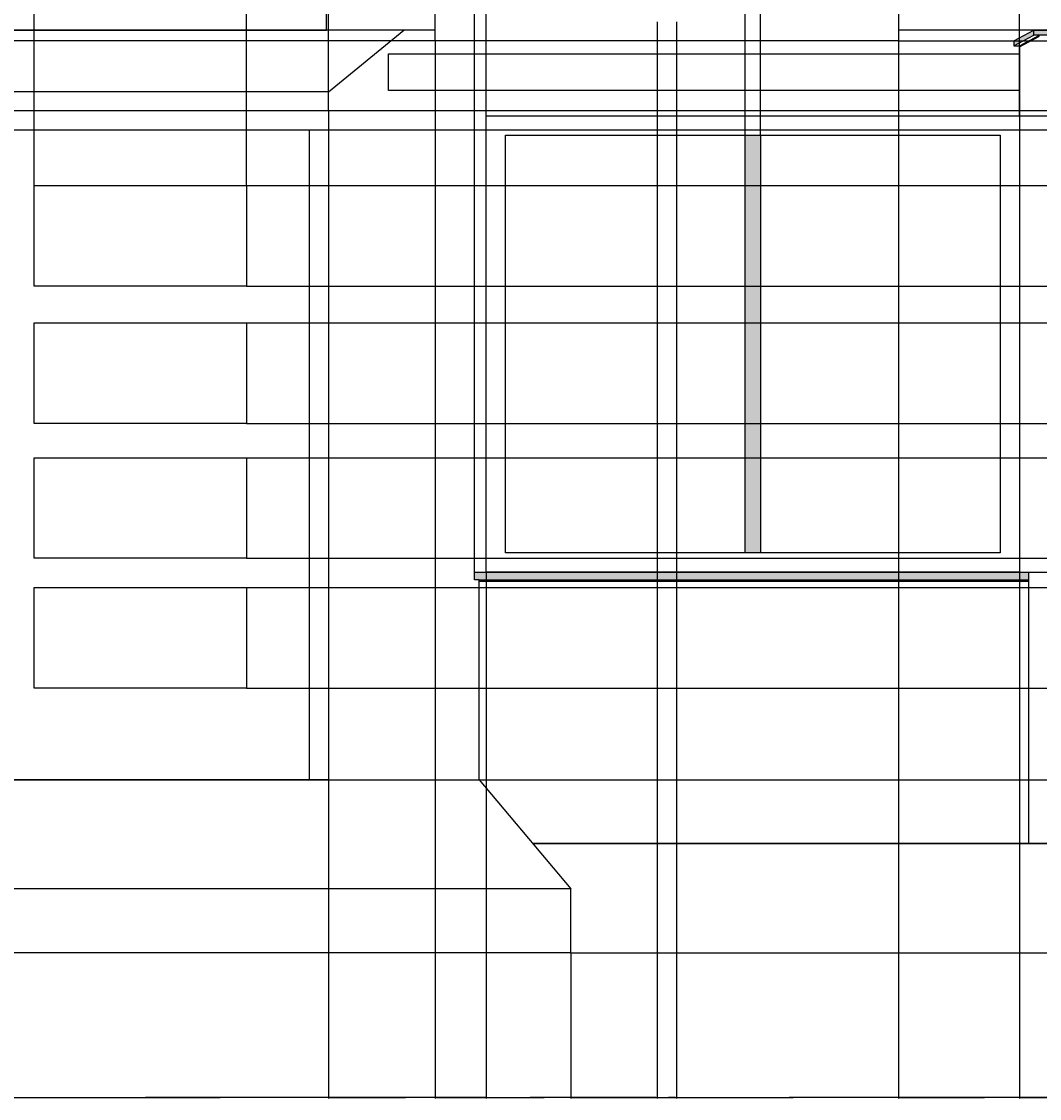
# Model space of a CAD drawing. Units: millimetres. Extents: x 171 to 1599, y 973 to 1509.
# Tile 5 of 7: x 1235 to 1445, y 973 to 1196. Entities that reach past the tile are written whole.
import ezdxf

# ---------------------------------------------------------------- set-up
doc = ezdxf.new("R2010")
doc.units = ezdxf.units.MM
for name, color, linetype, lineweight in [('A-ANNO-DIMS', 2, 'Continuous', 18), ('A-ELEV', 7, 'Continuous', 25), ('A-ELEV-FILL', 252, 'Continuous', 13)]:
    doc.layers.add(name, color=color, linetype=linetype, lineweight=lineweight)
doc.styles.get("Standard").update_dxf_attribs({"font": 'arial.ttf'})
doc.dimstyles.get("Standard").update_dxf_attribs({"dimtxt": 0.18, "dimasz": 0.18, "dimexe": 0.18, "dimexo": 0.0625, "dimgap": 0.09, "dimtad": 0, "dimtih": 1, "dimtoh": 1, "dimdec": 1, "dimzin": 0, "dimdsep": 46, "dimlunit": 3, "dimtxsty": 'Standard', "dimcen": 0.09, "dimadec": 0, "dimazin": 0, "dimtfac": 1, "dimtdec": 1, "dimtofl": 0, "dimtmove": 0, "dimatfit": 3, "dimfxl": 1, "dimtolj": 1, "dimtzin": 0, "dimarcsym": 0})

# ---------------------------------------------------------------- blocks, each defined once
blk = doc.blocks.new('*D1')
at = {"layer": 'A-ANNO-DIMS', "color": 0, "lineweight": -2, "transparency": 16777216}
for p, q in [((980.93, 1194.55), (980.93, 1508.31)), ((981.11, 1508.13), (1274.61, 1508.13)), ((1568.85, 1508.13), (1275.36, 1508.13)), ((1569.03, 1215.31), (1569.03, 1508.31))]:
    blk.add_line(p, q, dxfattribs=at)
at = {"layer": 'A-ANNO-DIMS', "color": 0, "transparency": 16777216}
for points in [[(981.11, 1508.16), (981.11, 1508.1), (980.93, 1508.13)], [(1568.85, 1508.16), (1568.85, 1508.1), (1569.03, 1508.13)]]:
    blk.add_solid(points, dxfattribs=at)
at = {"layer": 'Defpoints', "color": 0, "transparency": 16777216}
for p in [(1569.03, 1508.13), (1569.03, 1215.25), (980.93, 1194.49)]:
    blk.add_point(p, dxfattribs=at)
at = {"layer": 'A-ANNO-DIMS', "color": 0, "transparency": 16777216, "insert": (1274.98, 1508.13), "char_height": 0.18, "attachment_point": 5}
blk.add_mtext('\\A1;588.1', dxfattribs=at)
blk = doc.blocks.new('*D2')
at = {"layer": 'A-ANNO-DIMS', "color": 0, "lineweight": -2, "transparency": 16777216}
for p, q in [((1043.70287, 1478.130098), (1599.212656, 1478.130098)), ((1599.032656, 1477.950098), (1599.032656, 1240.959874)), ((1599.032656, 1003.60965), (1599.032656, 1240.599874)), ((1348.449149, 1003.42965), (1599.212656, 1003.42965))]:
    blk.add_line(p, q, dxfattribs=at)
at = {"layer": 'A-ANNO-DIMS', "color": 0, "transparency": 16777216}
for points in [[(1599.002656, 1477.950098), (1599.062656, 1477.950098), (1599.032656, 1478.130098)], [(1599.002656, 1003.60965), (1599.062656, 1003.60965), (1599.032656, 1003.42965)]]:
    blk.add_solid(points, dxfattribs=at)
at = {"layer": 'Defpoints', "color": 0, "transparency": 16777216}
for p in [(1043.64037, 1478.130098), (1599.032656, 1478.130098), (1348.386649, 1003.42965)]:
    blk.add_point(p, dxfattribs=at)
at = {"layer": 'A-ANNO-DIMS', "color": 0, "transparency": 16777216, "insert": (1599.032656, 1240.779874), "char_height": 0.18, "attachment_point": 5}
blk.add_mtext('\\A1;474.7', dxfattribs=at)
blk = doc.blocks.new('*D6')
at = {"layer": 'A-ANNO-DIMS', "color": 0, "lineweight": -2, "transparency": 16777216}
for p, q in [((1221.72, 1039.19), (1221.72, 973.25)), ((1298.24, 1039.19), (1298.24, 973.25)), ((1221.9, 973.43), (1259.59, 973.43)), ((1298.06, 973.43), (1260.37, 973.43))]:
    blk.add_line(p, q, dxfattribs=at)
at = {"layer": 'A-ANNO-DIMS', "color": 0, "transparency": 16777216}
for points in [[(1221.9, 973.46), (1221.9, 973.4), (1221.72, 973.43)], [(1298.06, 973.46), (1298.06, 973.4), (1298.24, 973.43)]]:
    blk.add_solid(points, dxfattribs=at)
at = {"layer": 'Defpoints', "color": 0, "transparency": 16777216}
for p in [(1221.72, 1039.25), (1298.24, 1039.25), (1298.24, 973.43)]:
    blk.add_point(p, dxfattribs=at)
at = {"layer": 'A-ANNO-DIMS', "color": 0, "transparency": 16777216, "insert": (1259.98, 973.43), "char_height": 0.18, "attachment_point": 5}
blk.add_mtext('\\A1;76.52', dxfattribs=at)
blk = doc.blocks.new('*D7')
at = {"layer": 'A-ANNO-DIMS', "color": 0, "lineweight": -2, "transparency": 16777216}
for p, q in [((1330.9, 1082.17), (1330.9, 973.25)), ((1298.24, 1039.19), (1298.24, 973.25)), ((1298.42, 973.43), (1314.17, 973.43)), ((1330.72, 973.43), (1314.96, 973.43))]:
    blk.add_line(p, q, dxfattribs=at)
at = {"layer": 'A-ANNO-DIMS', "color": 0, "transparency": 16777216}
for points in [[(1298.42, 973.46), (1298.42, 973.4), (1298.24, 973.43)], [(1330.72, 973.46), (1330.72, 973.4), (1330.9, 973.43)]]:
    blk.add_solid(points, dxfattribs=at)
at = {"layer": 'Defpoints', "color": 0, "transparency": 16777216}
for p in [(1330.9, 1082.23), (1298.24, 1039.25), (1330.9, 973.43)]:
    blk.add_point(p, dxfattribs=at)
at = {"layer": 'A-ANNO-DIMS', "color": 0, "transparency": 16777216, "insert": (1314.57, 973.43), "char_height": 0.18, "attachment_point": 5}
blk.add_mtext('\\A1;32.66', dxfattribs=at)
blk = doc.blocks.new('*D8')
at = {"layer": 'A-ANNO-DIMS', "color": 0, "lineweight": -2, "transparency": 16777216}
for p, q in [((1330.9, 1082.17), (1330.9, 973.25)), ((1348.39, 1003.37), (1348.39, 973.25)), ((1331.08, 973.43), (1339.26, 973.43)), ((1348.21, 973.43), (1340.03, 973.43))]:
    blk.add_line(p, q, dxfattribs=at)
at = {"layer": 'A-ANNO-DIMS', "color": 0, "transparency": 16777216}
for points in [[(1331.08, 973.46), (1331.08, 973.4), (1330.9, 973.43)], [(1348.21, 973.46), (1348.21, 973.4), (1348.39, 973.43)]]:
    blk.add_solid(points, dxfattribs=at)
at = {"layer": 'Defpoints', "color": 0, "transparency": 16777216}
for p in [(1330.9, 1082.23), (1348.39, 1003.43), (1348.39, 973.43)]:
    blk.add_point(p, dxfattribs=at)
at = {"layer": 'A-ANNO-DIMS', "color": 0, "transparency": 16777216, "insert": (1339.64, 973.43), "char_height": 0.18, "attachment_point": 5}
blk.add_mtext('\\A1;17.49', dxfattribs=at)
blk = doc.blocks.new('*D9')
at = {"layer": 'A-ANNO-DIMS', "color": 0, "lineweight": -2, "transparency": 16777216}
for p, q in [((1441.28, 1082.17), (1441.28, 973.25)), ((1348.39, 1003.37), (1348.39, 973.25)), ((1348.57, 973.43), (1394.44, 973.43)), ((1441.1, 973.43), (1395.23, 973.43))]:
    blk.add_line(p, q, dxfattribs=at)
at = {"layer": 'A-ANNO-DIMS', "color": 0, "transparency": 16777216}
for points in [[(1348.57, 973.46), (1348.57, 973.4), (1348.39, 973.43)], [(1441.1, 973.46), (1441.1, 973.4), (1441.28, 973.43)]]:
    blk.add_solid(points, dxfattribs=at)
at = {"layer": 'Defpoints', "color": 0, "transparency": 16777216}
for p in [(1441.28, 1082.23), (1348.39, 1003.43), (1441.28, 973.43)]:
    blk.add_point(p, dxfattribs=at)
at = {"layer": 'A-ANNO-DIMS', "color": 0, "transparency": 16777216, "insert": (1394.83, 973.43), "char_height": 0.18, "attachment_point": 5}
blk.add_mtext('\\A1;92.89', dxfattribs=at)
blk = doc.blocks.new('*D10')
at = {"layer": 'A-ANNO-DIMS', "color": 0, "lineweight": -2, "transparency": 16777216}
for p, q in [((1441.28, 1082.17), (1441.28, 973.25)), ((1504.77, 1026.01), (1504.77, 973.25)), ((1441.46, 973.43), (1472.63, 973.43)), ((1504.59, 973.43), (1473.42, 973.43))]:
    blk.add_line(p, q, dxfattribs=at)
at = {"layer": 'A-ANNO-DIMS', "color": 0, "transparency": 16777216}
for points in [[(1441.46, 973.46), (1441.46, 973.4), (1441.28, 973.43)], [(1504.59, 973.46), (1504.59, 973.4), (1504.77, 973.43)]]:
    blk.add_solid(points, dxfattribs=at)
at = {"layer": 'Defpoints', "color": 0, "transparency": 16777216}
for p in [(1441.28, 1082.23), (1504.77, 1026.08), (1504.77, 973.43)]:
    blk.add_point(p, dxfattribs=at)
at = {"layer": 'A-ANNO-DIMS', "color": 0, "transparency": 16777216, "insert": (1473.02, 973.43), "char_height": 0.18, "attachment_point": 5}
blk.add_mtext('\\A1;63.49', dxfattribs=at)
blk = doc.blocks.new('*D54')
at = {"layer": 'A-ANNO-DIMS', "color": 0, "lineweight": -2, "transparency": 16777216}
for p, q in [((1232.1, 1203.73), (1232.1, 973.25)), ((1320.32, 1192.2), (1320.32, 973.25)), ((1232.28, 973.43), (1275.82, 973.43)), ((1320.14, 973.43), (1276.6, 973.43))]:
    blk.add_line(p, q, dxfattribs=at)
at = {"layer": 'A-ANNO-DIMS', "color": 0, "transparency": 16777216}
for points in [[(1232.28, 973.46), (1232.28, 973.4), (1232.1, 973.43)], [(1320.14, 973.46), (1320.14, 973.4), (1320.32, 973.43)]]:
    blk.add_solid(points, dxfattribs=at)
at = {"layer": 'Defpoints', "color": 0, "transparency": 16777216}
for p in [(1232.1, 1203.79), (1320.32, 1192.27), (1320.32, 973.43)]:
    blk.add_point(p, dxfattribs=at)
at = {"layer": 'A-ANNO-DIMS', "color": 0, "transparency": 16777216, "insert": (1276.21, 973.43), "char_height": 0.18, "attachment_point": 5}
blk.add_mtext('\\A1;88.22', dxfattribs=at)
blk = doc.blocks.new('*D55')
at = {"layer": 'A-ANNO-DIMS', "color": 0, "lineweight": -2, "transparency": 16777216}
for p, q in [((1366.27, 1196.2), (1366.27, 973.25)), ((1320.32, 1192.2), (1320.32, 973.25)), ((1320.5, 973.43), (1342.9, 973.43)), ((1366.09, 973.43), (1343.69, 973.43))]:
    blk.add_line(p, q, dxfattribs=at)
at = {"layer": 'A-ANNO-DIMS', "color": 0, "transparency": 16777216}
for points in [[(1320.5, 973.46), (1320.5, 973.4), (1320.32, 973.43)], [(1366.09, 973.46), (1366.09, 973.4), (1366.27, 973.43)]]:
    blk.add_solid(points, dxfattribs=at)
at = {"layer": 'Defpoints', "color": 0, "transparency": 16777216}
for p in [(1366.27, 1196.27), (1320.32, 1192.27), (1366.27, 973.43)]:
    blk.add_point(p, dxfattribs=at)
at = {"layer": 'A-ANNO-DIMS', "color": 0, "transparency": 16777216, "insert": (1343.3, 973.43), "char_height": 0.18, "attachment_point": 5}
blk.add_mtext('\\A1;45.95', dxfattribs=at)
blk = doc.blocks.new('*D56')
at = {"layer": 'A-ANNO-DIMS', "color": 0, "lineweight": -2, "transparency": 16777216}
for p, q in [((1366.27, 1196.2), (1366.27, 973.25)), ((1370.27, 1196.2), (1370.27, 973.25)), ((1366.45, 973.43), (1367.94, 973.43)), ((1370.09, 973.43), (1368.6, 973.43))]:
    blk.add_line(p, q, dxfattribs=at)
at = {"layer": 'A-ANNO-DIMS', "color": 0, "transparency": 16777216}
for points in [[(1366.45, 973.46), (1366.45, 973.4), (1366.27, 973.43)], [(1370.09, 973.46), (1370.09, 973.4), (1370.27, 973.43)]]:
    blk.add_solid(points, dxfattribs=at)
at = {"layer": 'Defpoints', "color": 0, "transparency": 16777216}
for p in [(1366.27, 1196.27), (1370.27, 1196.27), (1370.27, 973.43)]:
    blk.add_point(p, dxfattribs=at)
at = {"layer": 'A-ANNO-DIMS', "color": 0, "transparency": 16777216, "insert": (1368.27, 973.43), "char_height": 0.18, "attachment_point": 5}
blk.add_mtext('\\A1;4.00', dxfattribs=at)
blk = doc.blocks.new('*D57')
at = {"layer": 'A-ANNO-DIMS', "color": 0, "lineweight": -2, "transparency": 16777216}
for p, q in [((1370.27, 1196.2), (1370.27, 973.25)), ((1416.22, 1192.2), (1416.22, 973.25)), ((1370.45, 973.43), (1392.85, 973.43)), ((1416.04, 973.43), (1393.64, 973.43))]:
    blk.add_line(p, q, dxfattribs=at)
at = {"layer": 'A-ANNO-DIMS', "color": 0, "transparency": 16777216}
for points in [[(1370.45, 973.46), (1370.45, 973.4), (1370.27, 973.43)], [(1416.04, 973.46), (1416.04, 973.4), (1416.22, 973.43)]]:
    blk.add_solid(points, dxfattribs=at)
at = {"layer": 'Defpoints', "color": 0, "transparency": 16777216}
for p in [(1370.27, 1196.27), (1416.22, 1192.27), (1416.22, 973.43)]:
    blk.add_point(p, dxfattribs=at)
at = {"layer": 'A-ANNO-DIMS', "color": 0, "transparency": 16777216, "insert": (1393.25, 973.43), "char_height": 0.18, "attachment_point": 5}
blk.add_mtext('\\A1;45.95', dxfattribs=at)
blk = doc.blocks.new('*D58')
at = {"layer": 'A-ANNO-DIMS', "color": 0, "lineweight": -2, "transparency": 16777216}
for p, q in [((1452.86, 1194.43), (1452.86, 973.25)), ((1416.22, 1192.2), (1416.22, 973.25)), ((1416.4, 973.43), (1434.08, 973.43)), ((1452.68, 973.43), (1435, 973.43))]:
    blk.add_line(p, q, dxfattribs=at)
at = {"layer": 'A-ANNO-DIMS', "color": 0, "transparency": 16777216}
for points in [[(1416.4, 973.46), (1416.4, 973.4), (1416.22, 973.43)], [(1452.68, 973.46), (1452.68, 973.4), (1452.86, 973.43)]]:
    blk.add_solid(points, dxfattribs=at)
at = {"layer": 'Defpoints', "color": 0, "transparency": 16777216}
for p in [(1452.86, 1194.49), (1416.22, 1192.27), (1452.86, 973.43)]:
    blk.add_point(p, dxfattribs=at)
at = {"layer": 'A-ANNO-DIMS', "color": 0, "transparency": 16777216, "insert": (1434.54, 973.43), "char_height": 0.18, "attachment_point": 5}
blk.add_mtext('\\A1;36.636', dxfattribs=at)
blk = doc.blocks.new('*D61')
at = {"layer": 'A-ANNO-DIMS', "color": 0, "lineweight": -2, "transparency": 16777216}
for p, q in [((1320.26, 1345.85), (950.75, 1345.85)), ((950.93, 1345.67), (950.93, 1269.24)), ((950.93, 1192.45), (950.93, 1268.88)), ((1320.26, 1192.27), (950.75, 1192.27))]:
    blk.add_line(p, q, dxfattribs=at)
at = {"layer": 'A-ANNO-DIMS', "color": 0, "transparency": 16777216}
for points in [[(950.9, 1345.67), (950.96, 1345.67), (950.93, 1345.85)], [(950.9, 1192.45), (950.96, 1192.45), (950.93, 1192.27)]]:
    blk.add_solid(points, dxfattribs=at)
at = {"layer": 'Defpoints', "color": 0, "transparency": 16777216}
for p in [(950.93, 1345.85), (1320.32, 1345.85), (1320.32, 1192.27)]:
    blk.add_point(p, dxfattribs=at)
at = {"layer": 'A-ANNO-DIMS', "color": 0, "transparency": 16777216, "insert": (950.93, 1269.06), "char_height": 0.18, "attachment_point": 5}
blk.add_mtext('\\A1;153.59', dxfattribs=at)
blk = doc.blocks.new('*D62')
at = {"layer": 'A-ANNO-DIMS', "color": 0, "lineweight": -2, "transparency": 16777216}
for p, q in [((1416.28, 1290.48), (1599.21, 1290.48)), ((1599.03, 1290.3), (1599.03, 1241.56)), ((1599.03, 1192.45), (1599.03, 1241.19)), ((1416.28, 1192.27), (1599.21, 1192.27))]:
    blk.add_line(p, q, dxfattribs=at)
at = {"layer": 'A-ANNO-DIMS', "color": 0, "transparency": 16777216}
for points in [[(1599, 1290.3), (1599.06, 1290.3), (1599.03, 1290.48)], [(1599, 1192.45), (1599.06, 1192.45), (1599.03, 1192.27)]]:
    blk.add_solid(points, dxfattribs=at)
at = {"layer": 'Defpoints', "color": 0, "transparency": 16777216}
for p in [(1416.22, 1290.48), (1599.03, 1290.48), (1416.22, 1192.27)]:
    blk.add_point(p, dxfattribs=at)
at = {"layer": 'A-ANNO-DIMS', "color": 0, "transparency": 16777216, "insert": (1599.03, 1241.38), "char_height": 0.18, "attachment_point": 5}
blk.add_mtext('\\A1;98.22', dxfattribs=at)
blk = doc.blocks.new('*D73')
at = {"layer": 'A-ANNO-DIMS', "color": 0, "lineweight": -2, "transparency": 16777216}
for p, q in [((1231.46, 1114.32), (1231.46, 1508.31)), ((1231.64, 1508.13), (1234.06, 1508.13)), ((1237.13, 1508.13), (1234.71, 1508.13)), ((1237.31, 1162.35), (1237.31, 1508.31))]:
    blk.add_line(p, q, dxfattribs=at)
at = {"layer": 'A-ANNO-DIMS', "color": 0, "transparency": 16777216}
for points in [[(1231.64, 1508.16), (1231.64, 1508.1), (1231.46, 1508.13)], [(1237.13, 1508.16), (1237.13, 1508.1), (1237.31, 1508.13)]]:
    blk.add_solid(points, dxfattribs=at)
at = {"layer": 'Defpoints', "color": 0, "transparency": 16777216}
for p in [(1237.31, 1508.13), (1237.31, 1162.29), (1231.46, 1114.25)]:
    blk.add_point(p, dxfattribs=at)
at = {"layer": 'A-ANNO-DIMS', "color": 0, "transparency": 16777216, "insert": (1234.38, 1508.13), "char_height": 0.18, "attachment_point": 5}
blk.add_mtext('\\A1;5.85', dxfattribs=at)
blk = doc.blocks.new('*D74')
at = {"layer": 'A-ANNO-DIMS', "color": 0, "lineweight": -2, "transparency": 16777216}
for p, q in [((1237.31, 1162.35), (1237.31, 1508.31)), ((1237.49, 1508.13), (1258.88, 1508.13)), ((1281.06, 1508.13), (1259.67, 1508.13)), ((1281.24, 1162.35), (1281.24, 1508.31))]:
    blk.add_line(p, q, dxfattribs=at)
at = {"layer": 'A-ANNO-DIMS', "color": 0, "transparency": 16777216}
for points in [[(1237.49, 1508.16), (1237.49, 1508.1), (1237.31, 1508.13)], [(1281.06, 1508.16), (1281.06, 1508.1), (1281.24, 1508.13)]]:
    blk.add_solid(points, dxfattribs=at)
at = {"layer": 'Defpoints', "color": 0, "transparency": 16777216}
for p in [(1281.24, 1508.13), (1237.31, 1162.29), (1281.24, 1162.29)]:
    blk.add_point(p, dxfattribs=at)
at = {"layer": 'A-ANNO-DIMS', "color": 0, "transparency": 16777216, "insert": (1259.27, 1508.13), "char_height": 0.18, "attachment_point": 5}
blk.add_mtext('\\A1;43.93', dxfattribs=at)
blk = doc.blocks.new('*D75')
at = {"layer": 'A-ANNO-DIMS', "color": 0, "lineweight": -2, "transparency": 16777216}
for p, q in [((1281.24, 1162.35), (1281.24, 1508.31)), ((1281.42, 1508.13), (1289.28, 1508.13)), ((1298.06, 1508.13), (1290.19, 1508.13)), ((1298.24, 1177.93), (1298.24, 1508.31))]:
    blk.add_line(p, q, dxfattribs=at)
at = {"layer": 'A-ANNO-DIMS', "color": 0, "transparency": 16777216}
for points in [[(1281.42, 1508.16), (1281.42, 1508.1), (1281.24, 1508.13)], [(1298.06, 1508.16), (1298.06, 1508.1), (1298.24, 1508.13)]]:
    blk.add_solid(points, dxfattribs=at)
at = {"layer": 'Defpoints', "color": 0, "transparency": 16777216}
for p in [(1298.24, 1508.13), (1298.24, 1177.87), (1281.24, 1162.29)]:
    blk.add_point(p, dxfattribs=at)
at = {"layer": 'A-ANNO-DIMS', "color": 0, "transparency": 16777216, "insert": (1289.74, 1508.13), "char_height": 0.18, "attachment_point": 5}
blk.add_mtext('\\A1;16.995', dxfattribs=at)
blk = doc.blocks.new('*D76')
at = {"layer": 'A-ANNO-DIMS', "color": 0, "lineweight": -2, "transparency": 16777216}
for p, q in [((1298.24, 1177.93), (1298.24, 1508.31)), ((1298.42, 1508.13), (1312.96, 1508.13)), ((1328.29, 1508.13), (1313.75, 1508.13)), ((1328.47, 1082.3), (1328.47, 1508.31))]:
    blk.add_line(p, q, dxfattribs=at)
at = {"layer": 'A-ANNO-DIMS', "color": 0, "transparency": 16777216}
for points in [[(1298.42, 1508.16), (1298.42, 1508.1), (1298.24, 1508.13)], [(1328.29, 1508.16), (1328.29, 1508.1), (1328.47, 1508.13)]]:
    blk.add_solid(points, dxfattribs=at)
at = {"layer": 'Defpoints', "color": 0, "transparency": 16777216}
for p in [(1328.47, 1508.13), (1298.24, 1177.87), (1328.47, 1082.23)]:
    blk.add_point(p, dxfattribs=at)
at = {"layer": 'A-ANNO-DIMS', "color": 0, "transparency": 16777216, "insert": (1313.36, 1508.13), "char_height": 0.18, "attachment_point": 5}
blk.add_mtext('\\A1;30.24', dxfattribs=at)
blk = doc.blocks.new('*D77')
at = {"layer": 'A-ANNO-DIMS', "color": 0, "lineweight": -2, "transparency": 16777216}
for p, q in [((1328.47, 1082.3), (1328.47, 1508.31)), ((1328.65, 1508.13), (1329.29, 1508.13)), ((1330.72, 1508.13), (1330.08, 1508.13)), ((1330.9, 1176.81), (1330.9, 1508.31))]:
    blk.add_line(p, q, dxfattribs=at)
at = {"layer": 'A-ANNO-DIMS', "color": 0, "transparency": 16777216}
for points in [[(1328.65, 1508.16), (1328.65, 1508.1), (1328.47, 1508.13)], [(1330.72, 1508.16), (1330.72, 1508.1), (1330.9, 1508.13)]]:
    blk.add_solid(points, dxfattribs=at)
at = {"layer": 'Defpoints', "color": 0, "transparency": 16777216}
for p in [(1330.9, 1508.13), (1330.9, 1176.74), (1328.47, 1082.23)]:
    blk.add_point(p, dxfattribs=at)
at = {"layer": 'A-ANNO-DIMS', "color": 0, "transparency": 16777216, "insert": (1329.69, 1508.13), "char_height": 0.18, "attachment_point": 5}
blk.add_mtext('\\A1;2.423', dxfattribs=at)
blk = doc.blocks.new('*D78')
at = {"layer": 'A-ANNO-DIMS', "color": 0, "lineweight": -2, "transparency": 16777216}
for p, q in [((1330.9, 1176.81), (1330.9, 1508.31)), ((1331.08, 1508.13), (1357.29, 1508.13)), ((1384.29, 1508.13), (1358.08, 1508.13)), ((1384.47, 1172.81), (1384.47, 1508.31))]:
    blk.add_line(p, q, dxfattribs=at)
at = {"layer": 'A-ANNO-DIMS', "color": 0, "transparency": 16777216}
for points in [[(1331.08, 1508.16), (1331.08, 1508.1), (1330.9, 1508.13)], [(1384.29, 1508.16), (1384.29, 1508.1), (1384.47, 1508.13)]]:
    blk.add_solid(points, dxfattribs=at)
at = {"layer": 'Defpoints', "color": 0, "transparency": 16777216}
for p in [(1384.47, 1508.13), (1330.9, 1176.74), (1384.47, 1172.74)]:
    blk.add_point(p, dxfattribs=at)
at = {"layer": 'A-ANNO-DIMS', "color": 0, "transparency": 16777216, "insert": (1357.69, 1508.13), "char_height": 0.18, "attachment_point": 5}
blk.add_mtext('\\A1;53.58', dxfattribs=at)
blk = doc.blocks.new('*D79')
at = {"layer": 'A-ANNO-DIMS', "color": 0, "lineweight": -2, "transparency": 16777216}
for p, q in [((1384.47, 1172.81), (1384.47, 1508.31)), ((1384.65, 1508.13), (1385.69, 1508.13)), ((1387.52, 1508.13), (1386.48, 1508.13)), ((1387.7, 1172.81), (1387.7, 1508.31))]:
    blk.add_line(p, q, dxfattribs=at)
at = {"layer": 'A-ANNO-DIMS', "color": 0, "transparency": 16777216}
for points in [[(1384.65, 1508.16), (1384.65, 1508.1), (1384.47, 1508.13)], [(1387.52, 1508.16), (1387.52, 1508.1), (1387.7, 1508.13)]]:
    blk.add_solid(points, dxfattribs=at)
at = {"layer": 'Defpoints', "color": 0, "transparency": 16777216}
for p in [(1387.7, 1508.13), (1384.47, 1172.74), (1387.7, 1172.74)]:
    blk.add_point(p, dxfattribs=at)
at = {"layer": 'A-ANNO-DIMS', "color": 0, "transparency": 16777216, "insert": (1386.09, 1508.13), "char_height": 0.18, "attachment_point": 5}
blk.add_mtext('\\A1;3.224', dxfattribs=at)
blk = doc.blocks.new('*D80')
at = {"layer": 'A-ANNO-DIMS', "color": 0, "lineweight": -2, "transparency": 16777216}
for p, q in [((1387.7, 1172.81), (1387.7, 1508.31)), ((1387.88, 1508.13), (1414.09, 1508.13)), ((1441.1, 1508.13), (1414.88, 1508.13)), ((1441.28, 1176.81), (1441.28, 1508.31))]:
    blk.add_line(p, q, dxfattribs=at)
at = {"layer": 'A-ANNO-DIMS', "color": 0, "transparency": 16777216}
for points in [[(1387.88, 1508.16), (1387.88, 1508.1), (1387.7, 1508.13)], [(1441.1, 1508.16), (1441.1, 1508.1), (1441.28, 1508.13)]]:
    blk.add_solid(points, dxfattribs=at)
at = {"layer": 'Defpoints', "color": 0, "transparency": 16777216}
for p in [(1441.28, 1508.13), (1441.28, 1176.74), (1387.7, 1172.74)]:
    blk.add_point(p, dxfattribs=at)
at = {"layer": 'A-ANNO-DIMS', "color": 0, "transparency": 16777216, "insert": (1414.49, 1508.13), "char_height": 0.18, "attachment_point": 5}
blk.add_mtext('\\A1;53.58', dxfattribs=at)
blk = doc.blocks.new('*D86')
at = {"layer": 'A-ANNO-DIMS', "color": 0, "lineweight": -2, "transparency": 16777216}
for p, q in [((1441.34, 1176.74), (1599.21, 1176.74)), ((1599.03, 1176.56), (1599.03, 1129.67)), ((1599.03, 1082.41), (1599.03, 1129.31)), ((1441.34, 1082.23), (1599.21, 1082.23))]:
    blk.add_line(p, q, dxfattribs=at)
at = {"layer": 'A-ANNO-DIMS', "color": 0, "transparency": 16777216}
for points in [[(1599, 1176.56), (1599.06, 1176.56), (1599.03, 1176.74)], [(1599, 1082.41), (1599.06, 1082.41), (1599.03, 1082.23)]]:
    blk.add_solid(points, dxfattribs=at)
at = {"layer": 'Defpoints', "color": 0, "transparency": 16777216}
for p in [(1441.28, 1176.74), (1599.03, 1176.74), (1441.28, 1082.23)]:
    blk.add_point(p, dxfattribs=at)
at = {"layer": 'A-ANNO-DIMS', "color": 0, "transparency": 16777216, "insert": (1599.03, 1129.49), "char_height": 0.18, "attachment_point": 5}
blk.add_mtext('\\A1;94.51', dxfattribs=at)
blk = doc.blocks.new('*D87')
at = {"layer": 'A-ANNO-DIMS', "color": 0, "lineweight": -2, "transparency": 16777216}
for p, q in [((1281.3, 1058.21), (1599.21, 1058.21)), ((1599.03, 1058.03), (1599.03, 1048.91)), ((1599.03, 1039.43), (1599.03, 1048.55)), ((1294.3, 1039.25), (1599.21, 1039.25))]:
    blk.add_line(p, q, dxfattribs=at)
at = {"layer": 'A-ANNO-DIMS', "color": 0, "transparency": 16777216}
for points in [[(1599, 1058.03), (1599.06, 1058.03), (1599.03, 1058.21)], [(1599, 1039.43), (1599.06, 1039.43), (1599.03, 1039.25)]]:
    blk.add_solid(points, dxfattribs=at)
at = {"layer": 'Defpoints', "color": 0, "transparency": 16777216}
for p in [(1281.24, 1058.21), (1599.03, 1058.21), (1294.24, 1039.25)]:
    blk.add_point(p, dxfattribs=at)
at = {"layer": 'A-ANNO-DIMS', "color": 0, "transparency": 16777216, "insert": (1599.03, 1048.73), "char_height": 0.18, "attachment_point": 5}
blk.add_mtext('\\A1;18.956', dxfattribs=at)
blk = doc.blocks.new('*D88')
at = {"layer": 'A-ANNO-DIMS', "color": 0, "lineweight": -2, "transparency": 16777216}
for p, q in [((1281.3, 1079.04), (1599.21, 1079.04)), ((1599.03, 1078.86), (1599.03, 1068.8)), ((1599.03, 1058.39), (1599.03, 1068.44)), ((1281.3, 1058.21), (1599.21, 1058.21))]:
    blk.add_line(p, q, dxfattribs=at)
at = {"layer": 'A-ANNO-DIMS', "color": 0, "transparency": 16777216}
for points in [[(1599, 1078.86), (1599.06, 1078.86), (1599.03, 1079.04)], [(1599, 1058.39), (1599.06, 1058.39), (1599.03, 1058.21)]]:
    blk.add_solid(points, dxfattribs=at)
at = {"layer": 'Defpoints', "color": 0, "transparency": 16777216}
for p in [(1281.24, 1079.04), (1599.03, 1079.04), (1281.24, 1058.21)]:
    blk.add_point(p, dxfattribs=at)
at = {"layer": 'A-ANNO-DIMS', "color": 0, "transparency": 16777216, "insert": (1599.03, 1068.62), "char_height": 0.18, "attachment_point": 5}
blk.add_mtext('\\A1;20.833', dxfattribs=at)
blk = doc.blocks.new('*D89')
at = {"layer": 'A-ANNO-DIMS', "color": 0, "lineweight": -2, "transparency": 16777216}
for p, q in [((1281.3, 1085.12), (1599.21, 1085.12)), ((1599.03, 1084.94), (1599.03, 1082.26)), ((1599.03, 1079.22), (1599.03, 1081.9)), ((1281.3, 1079.04), (1599.21, 1079.04))]:
    blk.add_line(p, q, dxfattribs=at)
at = {"layer": 'A-ANNO-DIMS', "color": 0, "transparency": 16777216}
for points in [[(1599, 1084.94), (1599.06, 1084.94), (1599.03, 1085.12)], [(1599, 1079.22), (1599.06, 1079.22), (1599.03, 1079.04)]]:
    blk.add_solid(points, dxfattribs=at)
at = {"layer": 'Defpoints', "color": 0, "transparency": 16777216}
for p in [(1281.24, 1085.12), (1599.03, 1085.12), (1281.24, 1079.04)]:
    blk.add_point(p, dxfattribs=at)
at = {"layer": 'A-ANNO-DIMS', "color": 0, "transparency": 16777216, "insert": (1599.03, 1082.08), "char_height": 0.18, "attachment_point": 5}
blk.add_mtext('\\A1;6.079', dxfattribs=at)
blk = doc.blocks.new('*D90')
at = {"layer": 'A-ANNO-DIMS', "color": 0, "lineweight": -2, "transparency": 16777216}
for p, q in [((1281.3, 1105.95), (1599.21, 1105.95)), ((1599.03, 1105.77), (1599.03, 1095.72)), ((1599.03, 1085.3), (1599.03, 1095.35)), ((1281.3, 1085.12), (1599.21, 1085.12))]:
    blk.add_line(p, q, dxfattribs=at)
at = {"layer": 'A-ANNO-DIMS', "color": 0, "transparency": 16777216}
for points in [[(1599, 1105.77), (1599.06, 1105.77), (1599.03, 1105.95)], [(1599, 1085.3), (1599.06, 1085.3), (1599.03, 1085.12)]]:
    blk.add_solid(points, dxfattribs=at)
at = {"layer": 'Defpoints', "color": 0, "transparency": 16777216}
for p in [(1281.24, 1105.95), (1599.03, 1105.95), (1281.24, 1085.12)]:
    blk.add_point(p, dxfattribs=at)
at = {"layer": 'A-ANNO-DIMS', "color": 0, "transparency": 16777216, "insert": (1599.03, 1095.53), "char_height": 0.18, "attachment_point": 5}
blk.add_mtext('\\A1;20.833', dxfattribs=at)
blk = doc.blocks.new('*D91')
at = {"layer": 'A-ANNO-DIMS', "color": 0, "lineweight": -2, "transparency": 16777216}
for p, q in [((1281.3, 1113.05), (1599.21, 1113.05)), ((1599.03, 1112.87), (1599.03, 1109.68)), ((1599.03, 1106.13), (1599.03, 1109.32)), ((1281.3, 1105.95), (1599.21, 1105.95))]:
    blk.add_line(p, q, dxfattribs=at)
at = {"layer": 'A-ANNO-DIMS', "color": 0, "transparency": 16777216}
for points in [[(1599, 1112.87), (1599.06, 1112.87), (1599.03, 1113.05)], [(1599, 1106.13), (1599.06, 1106.13), (1599.03, 1105.95)]]:
    blk.add_solid(points, dxfattribs=at)
at = {"layer": 'Defpoints', "color": 0, "transparency": 16777216}
for p in [(1281.24, 1113.05), (1599.03, 1113.05), (1281.24, 1105.95)]:
    blk.add_point(p, dxfattribs=at)
at = {"layer": 'A-ANNO-DIMS', "color": 0, "transparency": 16777216, "insert": (1599.03, 1109.5), "char_height": 0.18, "attachment_point": 5}
blk.add_mtext('\\A1;7.102', dxfattribs=at)
blk = doc.blocks.new('*D92')
at = {"layer": 'A-ANNO-DIMS', "color": 0, "lineweight": -2, "transparency": 16777216}
for p, q in [((1281.3, 1133.89), (1599.21, 1133.89)), ((1599.03, 1133.71), (1599.03, 1123.65)), ((1599.03, 1113.23), (1599.03, 1123.29)), ((1281.3, 1113.05), (1599.21, 1113.05))]:
    blk.add_line(p, q, dxfattribs=at)
at = {"layer": 'A-ANNO-DIMS', "color": 0, "transparency": 16777216}
for points in [[(1599, 1133.71), (1599.06, 1133.71), (1599.03, 1133.89)], [(1599, 1113.23), (1599.06, 1113.23), (1599.03, 1113.05)]]:
    blk.add_solid(points, dxfattribs=at)
at = {"layer": 'Defpoints', "color": 0, "transparency": 16777216}
for p in [(1281.24, 1133.89), (1599.03, 1133.89), (1281.24, 1113.05)]:
    blk.add_point(p, dxfattribs=at)
at = {"layer": 'A-ANNO-DIMS', "color": 0, "transparency": 16777216, "insert": (1599.03, 1123.47), "char_height": 0.18, "attachment_point": 5}
blk.add_mtext('\\A1;20.833', dxfattribs=at)
blk = doc.blocks.new('*D93')
at = {"layer": 'A-ANNO-DIMS', "color": 0, "lineweight": -2, "transparency": 16777216}
for p, q in [((1281.3, 1141.45), (1599.21, 1141.45)), ((1599.03, 1141.27), (1599.03, 1137.85)), ((1599.03, 1134.07), (1599.03, 1137.49)), ((1281.3, 1133.89), (1599.21, 1133.89))]:
    blk.add_line(p, q, dxfattribs=at)
at = {"layer": 'A-ANNO-DIMS', "color": 0, "transparency": 16777216}
for points in [[(1599, 1141.27), (1599.06, 1141.27), (1599.03, 1141.45)], [(1599, 1134.07), (1599.06, 1134.07), (1599.03, 1133.89)]]:
    blk.add_solid(points, dxfattribs=at)
at = {"layer": 'Defpoints', "color": 0, "transparency": 16777216}
for p in [(1281.24, 1141.45), (1599.03, 1141.45), (1281.24, 1133.89)]:
    blk.add_point(p, dxfattribs=at)
at = {"layer": 'A-ANNO-DIMS', "color": 0, "transparency": 16777216, "insert": (1599.03, 1137.67), "char_height": 0.18, "attachment_point": 5}
blk.add_mtext('\\A1;7.567', dxfattribs=at)
blk = doc.blocks.new('*D94')
at = {"layer": 'A-ANNO-DIMS', "color": 0, "lineweight": -2, "transparency": 16777216}
for p, q in [((1281.3, 1162.29), (1599.21, 1162.29)), ((1599.03, 1162.11), (1599.03, 1152.05)), ((1599.03, 1141.63), (1599.03, 1151.69)), ((1281.3, 1141.45), (1599.21, 1141.45))]:
    blk.add_line(p, q, dxfattribs=at)
at = {"layer": 'A-ANNO-DIMS', "color": 0, "transparency": 16777216}
for points in [[(1599, 1162.11), (1599.06, 1162.11), (1599.03, 1162.29)], [(1599, 1141.63), (1599.06, 1141.63), (1599.03, 1141.45)]]:
    blk.add_solid(points, dxfattribs=at)
at = {"layer": 'Defpoints', "color": 0, "transparency": 16777216}
for p in [(1281.24, 1162.29), (1599.03, 1162.29), (1281.24, 1141.45)]:
    blk.add_point(p, dxfattribs=at)
at = {"layer": 'A-ANNO-DIMS', "color": 0, "transparency": 16777216, "insert": (1599.03, 1151.87), "char_height": 0.18, "attachment_point": 5}
blk.add_mtext('\\A1;20.833', dxfattribs=at)
blk = doc.blocks.new('*D95')
at = {"layer": 'A-ANNO-DIMS', "color": 0, "lineweight": -2, "transparency": 16777216}
for p, q in [((1294.3, 1173.87), (1599.21, 1173.87)), ((1599.03, 1173.69), (1599.03, 1168.26)), ((1599.03, 1162.47), (1599.03, 1167.9)), ((1281.3, 1162.29), (1599.21, 1162.29))]:
    blk.add_line(p, q, dxfattribs=at)
at = {"layer": 'A-ANNO-DIMS', "color": 0, "transparency": 16777216}
for points in [[(1599, 1173.69), (1599.06, 1173.69), (1599.03, 1173.87)], [(1599, 1162.47), (1599.06, 1162.47), (1599.03, 1162.29)]]:
    blk.add_solid(points, dxfattribs=at)
at = {"layer": 'Defpoints', "color": 0, "transparency": 16777216}
for p in [(1294.24, 1173.87), (1599.03, 1173.87), (1281.24, 1162.29)]:
    blk.add_point(p, dxfattribs=at)
at = {"layer": 'A-ANNO-DIMS', "color": 0, "transparency": 16777216, "insert": (1599.03, 1168.08), "char_height": 0.18, "attachment_point": 5}
blk.add_mtext('\\A1;11.587', dxfattribs=at)
blk = doc.blocks.new('*D96')
at = {"layer": 'A-ANNO-DIMS', "color": 0, "lineweight": -2, "transparency": 16777216}
for p, q in [((1298.3, 1177.87), (1599.21, 1177.87)), ((1599.03, 1177.69), (1599.03, 1176.05)), ((1599.03, 1174.05), (1599.03, 1175.69)), ((1294.3, 1173.87), (1599.21, 1173.87))]:
    blk.add_line(p, q, dxfattribs=at)
at = {"layer": 'A-ANNO-DIMS', "color": 0, "transparency": 16777216}
for points in [[(1599, 1177.69), (1599.06, 1177.69), (1599.03, 1177.87)], [(1599, 1174.05), (1599.06, 1174.05), (1599.03, 1173.87)]]:
    blk.add_solid(points, dxfattribs=at)
at = {"layer": 'Defpoints', "color": 0, "transparency": 16777216}
for p in [(1298.24, 1177.87), (1599.03, 1177.87), (1294.24, 1173.87)]:
    blk.add_point(p, dxfattribs=at)
at = {"layer": 'A-ANNO-DIMS', "color": 0, "transparency": 16777216, "insert": (1599.03, 1175.87), "char_height": 0.18, "attachment_point": 5}
blk.add_mtext('\\A1;4.00', dxfattribs=at)

msp = doc.modelspace()

# ---------------------------------------------------------------- hatches: boundary and pattern name
at = {"layer": 'A-ELEV-FILL'}
h = msp.add_hatch(color=256, dxfattribs=at)
h.dxf.hatch_style = 1
h.paths.add_polyline_path([(1182.7346, 1341.8717), (1108.8176, 1341.8717), (1108.8176, 1220.867), (1182.7346, 1220.867)])
h.paths.add_polyline_path([(1181.7346, 1221.867), (1109.8176, 1221.867), (1109.8176, 1340.8717), (1181.7346, 1340.8717)], flags=16)
h.paths.add_polyline_path([(1180.7346, 1339.8717), (1180.7346, 1282.2145), (1181.7346, 1282.2145), (1181.7346, 1280.5242), (1109.8176, 1280.5242), (1109.8176, 1282.2145), (1110.8176, 1282.2145), (1110.8176, 1339.8717)], flags=0)
h.paths.add_polyline_path([(1180.7346, 1279.5242), (1180.7346, 1222.867), (1110.8176, 1222.867), (1110.8176, 1279.5242)], flags=0)
h.paths.add_polyline_path([(1387.6984, 1172.7441), (1384.4743, 1172.7441), (1384.4743, 1086.2327), (1387.6984, 1086.2327)])
h = msp.add_hatch(color=256, dxfattribs=at)
h.dxf.hatch_style = 1
h.paths.add_polyline_path([(1507.6024, 1194.488), (1444.2789, 1194.488), (1444.2789, 1193.4707), (1507.6024, 1193.4707)])
h.paths.add_polyline_path([(1444.2789, 1193.4707), (1444.2789, 1194.488), (1440.129, 1192.267), (1440.129, 1191.2497)])
h = msp.add_hatch(color=256, dxfattribs=at)
h.dxf.hatch_style = 1
h.paths.add_polyline_path([(1057.1375, 1082.2327), (1051.6226, 1082.2327), (1051.6226, 1080.6718), (1057.1375, 1080.6718)])
h.paths.add_polyline_path([(1143.7, 1082.2327), (1057.1375, 1082.2327), (1057.1375, 1080.6718), (1143.7, 1080.6718)])
h.paths.add_polyline_path([(1509.9876, 1082.2327), (1504.7689, 1082.2327), (1504.7689, 1080.6718), (1509.0669, 1080.6718), (1509.9876, 1080.6718)])
h.paths.add_polyline_path([(1443.1972, 1082.2327), (1328.4737, 1082.2327), (1328.4737, 1080.6718), (1329.4402, 1080.6718), (1443.1972, 1080.6718)])

# ---------------------------------------------------------------- linework, layer by layer
at = {"layer": 'A-ELEV'}
for p, q in [((1320.3201, 1194.488), (980.9303, 1194.488)), ((1298.2363, 1181.6916), (1313.8358, 1194.488)), ((1444.2789, 1194.488), (1416.2216, 1194.488)), ((1440.129, 1192.267), (1444.2789, 1194.488)), ((1507.6024, 1194.488), (1440.129, 1194.488)), ((1440.129, 1191.2497), (1444.2789, 1193.4707)), ((1441.2762, 1191.2497), (1445.4261, 1193.4707)), ((1441.2762, 1191.0011), (1445.4261, 1193.222)), ((1440.129, 1192.267), (1440.129, 1191.2497)), ((1440.129, 1191.2497), (1441.2762, 1191.2497)), ((1441.2762, 1191.2497), (1441.2762, 1082.2327)), ((1443.1972, 1026.0387), (1443.1972, 1082.2327)), ((1329.4402, 1080.6718), (1329.4402, 1080.3893)), ((1329.4402, 1080.3893), (1443.1972, 1080.3893)), ((1340.5107, 1026.0387), (1509.0669, 1026.0387)), ((1348.3866, 1003.4297), (1348.3866, 1016.6402))]:
    msp.add_line(p, q, dxfattribs=at)
for points in [[(1416.2216, 1290.4846), (1416.2216, 1192.267), (1320.3201, 1192.267), (1320.3201, 1345.8534)], [(980.9303, 1194.488), (1297.8374, 1194.488), (1297.8374, 1203.7941), (980.9303, 1203.7941)], [(1064.505, 1177.8722), (1298.2363, 1177.8722), (1298.2363, 1181.6916), (1064.505, 1181.6916)], [(1225.7194, 1039.2493), (1225.7194, 1173.8722), (1294.2363, 1173.8722), (1294.2363, 1039.2493)], [(1384.4743, 1086.2327), (1384.4743, 1172.7441)], [(1387.6984, 1172.7441), (1387.6984, 1086.2327)], [(1329.4402, 1080.6718), (1328.4737, 1080.6718), (1328.4737, 1082.2327), (1443.1972, 1082.2327)], [(1329.4402, 1039.2493), (1329.4402, 1080.6718), (1443.1972, 1080.6718)], [(1504.7689, 1080.6718), (1509.0669, 1080.6718), (1509.0669, 1026.0387), (1340.5107, 1026.0387)], [(1329.4402, 1039.2493), (1348.3866, 1016.6402), (1013.0567, 1016.6402), (1029.0669, 1039.2493)], [(1029.0669, 1039.2493), (1329.4402, 1039.2493)], [(1348.3866, 1003.4297), (1013.0567, 1003.4297)]]:
    msp.add_lwpolyline(points, dxfattribs=at)
for points in [[(1507.6024, 1193.4707), (1444.2789, 1193.4707), (1444.2789, 1194.488), (1507.6024, 1194.488)], [(1441.2762, 1181.9686), (1310.6378, 1181.9686), (1310.6378, 1189.6048), (1441.2762, 1189.6048)], [(1298.2363, 1039.2493), (1221.7194, 1039.2493), (1221.7194, 1177.8722), (1298.2363, 1177.8722)], [(1441.2762, 1082.2327), (1330.8966, 1082.2327), (1330.8966, 1176.7441), (1441.2762, 1176.7441)], [(1437.2762, 1086.2327), (1334.8966, 1086.2327), (1334.8966, 1172.7441), (1437.2762, 1172.7441)], [(1281.2416, 1141.4523), (1237.3083, 1141.4523), (1237.3083, 1162.2854), (1281.2416, 1162.2854)], [(1281.2416, 1113.0519), (1237.3083, 1113.0519), (1237.3083, 1133.885), (1281.2416, 1133.885)], [(1281.2416, 1085.1172), (1237.3083, 1085.1172), (1237.3083, 1105.9503), (1281.2416, 1105.9503)], [(1281.2416, 1058.2052), (1237.3083, 1058.2052), (1237.3083, 1079.0383), (1281.2416, 1079.0383)]]:
    msp.add_lwpolyline(points, close=True, dxfattribs=at)

# ---------------------------------------------------------------- dimensions: what is measured, and where the dimension line sits
at = {"layer": 'A-ANNO-DIMS'}
for base, p1, p2, override, picture, middle in [((1569.0327, 1508.1301), (980.9303, 1194.488), (1569.0327, 1215.2519), {"dimdec": 1, "dimlfac": 1, "dimrnd": 0, "dimzin": 0, "dimdsep": 46, "dimlunit": 2}, '*D1', (1274.9815, 1508.1301)), ((1237.3083, 1508.1301), (1231.4586, 1114.2546), (1237.3083, 1162.2854), {"dimdec": 2, "dimlfac": 1, "dimrnd": 0, "dimzin": 0, "dimdsep": 46, "dimlunit": 2}, '*D73', (1234.3834, 1508.1301)), ((1281.2416, 1508.1301), (1237.3083, 1162.2854), (1281.2416, 1162.2854), {"dimdec": 2, "dimlfac": 1, "dimrnd": 0, "dimzin": 0, "dimdsep": 46, "dimlunit": 2}, '*D74', (1259.275, 1508.1301)), ((1298.2363, 1508.1301), (1281.2416, 1162.2854), (1298.2363, 1177.8722), {"dimdec": 3, "dimlfac": 1, "dimrnd": 0, "dimzin": 0, "dimdsep": 46, "dimlunit": 2}, '*D75', (1289.739, 1508.1301)), ((1328.4737, 1508.1301), (1298.2363, 1177.8722), (1328.4737, 1082.2327), {"dimdec": 2, "dimlfac": 1, "dimrnd": 0, "dimzin": 0, "dimdsep": 46, "dimlunit": 2}, '*D76', (1313.355, 1508.1301)), ((1330.8966, 1508.1301), (1328.4737, 1082.2327), (1330.8966, 1176.7441), {"dimdec": 3, "dimlfac": 1, "dimrnd": 0, "dimzin": 0, "dimdsep": 46, "dimlunit": 2}, '*D77', (1329.6852, 1508.1301)), ((1384.4743, 1508.1301), (1330.8966, 1176.7441), (1384.4743, 1172.7441), {"dimdec": 2, "dimlfac": 1, "dimrnd": 0, "dimzin": 0, "dimdsep": 46, "dimlunit": 2}, '*D78', (1357.6855, 1508.1301)), ((1387.6984, 1508.1301), (1384.4743, 1172.7441), (1387.6984, 1172.7441), {"dimdec": 3, "dimlfac": 1, "dimrnd": 0, "dimzin": 0, "dimdsep": 46, "dimlunit": 2}, '*D79', (1386.0864, 1508.1301)), ((1441.2762, 1508.1301), (1387.6984, 1172.7441), (1441.2762, 1176.7441), {"dimdec": 2, "dimlfac": 1, "dimrnd": 0, "dimzin": 0, "dimdsep": 46, "dimlunit": 2}, '*D80', (1414.4873, 1508.1301)), ((1320.3201, 973.4297), (1232.0993, 1203.7941), (1320.3201, 1192.267), {"dimdec": 2, "dimlfac": 1, "dimrnd": 0, "dimzin": 0, "dimdsep": 46, "dimlunit": 2}, '*D54', (1276.2097, 973.4297)), ((1366.2709, 973.4297), (1320.3201, 1192.267), (1366.2709, 1196.267), {"dimdec": 2, "dimlfac": 1, "dimrnd": 0, "dimzin": 0, "dimdsep": 46, "dimlunit": 2}, '*D55', (1343.2955, 973.4297)), ((1370.2709, 973.4297), (1366.2709, 1196.267), (1370.2709, 1196.267), {"dimdec": 2, "dimlfac": 1, "dimrnd": 0, "dimzin": 0, "dimdsep": 46, "dimlunit": 2}, '*D56', (1368.2709, 973.4297)), ((1416.2216, 973.4297), (1370.2709, 1196.267), (1416.2216, 1192.267), {"dimdec": 2, "dimlfac": 1, "dimrnd": 0, "dimzin": 0, "dimdsep": 46, "dimlunit": 2}, '*D57', (1393.2463, 973.4297)), ((1452.8572, 973.4297), (1416.2216, 1192.267), (1452.8572, 1194.488), {"dimdec": 3, "dimlfac": 1, "dimrnd": 0, "dimzin": 0, "dimdsep": 46, "dimlunit": 2}, '*D58', (1434.5394, 973.4297)), ((1330.8966, 973.4297), (1298.2363, 1039.2493), (1330.8966, 1082.2327), {"dimdec": 2, "dimlfac": 1, "dimrnd": 0, "dimzin": 0, "dimdsep": 46, "dimlunit": 2}, '*D7', (1314.5665, 973.4297)), ((1348.3866, 973.4297), (1330.8966, 1082.2327), (1348.3866, 1003.4297), {"dimdec": 2, "dimlfac": 1, "dimrnd": 0, "dimzin": 0, "dimdsep": 46, "dimlunit": 2}, '*D8', (1339.6416, 973.4297)), ((1441.2762, 973.4297), (1348.3866, 1003.4297), (1441.2762, 1082.2327), {"dimdec": 2, "dimlfac": 1, "dimrnd": 0, "dimzin": 0, "dimdsep": 46, "dimlunit": 2}, '*D9', (1394.8314, 973.4297)), ((1504.7689, 973.4297), (1441.2762, 1082.2327), (1504.7689, 1026.0766), {"dimdec": 2, "dimlfac": 1, "dimrnd": 0, "dimzin": 0, "dimdsep": 46, "dimlunit": 2}, '*D10', (1473.0225, 973.4297)), ((1298.2363, 973.4297), (1221.7194, 1039.2493), (1298.2363, 1039.2493), {"dimdec": 2, "dimlfac": 1, "dimrnd": 0, "dimzin": 0, "dimdsep": 46, "dimlunit": 2}, '*D6', (1259.9779, 973.4297))]:
    dim = msp.add_linear_dim(base=base, p1=p1, p2=p2, dimstyle='Standard', override=override, dxfattribs=at)
    dim.commit()
    dim.dimension.update_dxf_attribs({"geometry": picture, "text_midpoint": middle})
for base, p1, p2, override, picture, middle in [((1599.0327, 1478.1301), (1348.3866, 1003.4297), (1043.6404, 1478.1301), {"dimdec": 1, "dimlfac": 1, "dimrnd": 0, "dimzin": 0, "dimdsep": 46, "dimlunit": 2}, '*D2', (1599.0327, 1240.7799)), ((950.9303, 1345.8534), (1320.3201, 1192.267), (1320.3201, 1345.8534), {"dimdec": 2, "dimlfac": 1, "dimrnd": 0, "dimzin": 0, "dimdsep": 46, "dimlunit": 2}, '*D61', (950.9303, 1269.0602)), ((1599.0327, 1290.4846), (1416.2216, 1192.267), (1416.2216, 1290.4846), {"dimdec": 2, "dimlfac": 1, "dimrnd": 0, "dimzin": 0, "dimdsep": 46, "dimlunit": 2}, '*D62', (1599.0327, 1241.3758)), ((1599.0327, 1177.8722), (1294.2363, 1173.8722), (1298.2363, 1177.8722), {"dimdec": 2, "dimlfac": 1, "dimrnd": 0, "dimzin": 0, "dimdsep": 46, "dimlunit": 2}, '*D96', (1599.0327, 1175.8722)), ((1599.0327, 1176.7441), (1441.2762, 1082.2327), (1441.2762, 1176.7441), {"dimdec": 2, "dimlfac": 1, "dimrnd": 0, "dimzin": 0, "dimdsep": 46, "dimlunit": 2}, '*D86', (1599.0327, 1129.4884)), ((1599.0327, 1173.8722), (1281.2416, 1162.2854), (1294.2363, 1173.8722), {"dimdec": 3, "dimlfac": 1, "dimrnd": 0, "dimzin": 0, "dimdsep": 46, "dimlunit": 2}, '*D95', (1599.0327, 1168.0788)), ((1599.0327, 1162.2854), (1281.2416, 1141.4523), (1281.2416, 1162.2854), {"dimdec": 3, "dimlfac": 1, "dimrnd": 0, "dimzin": 0, "dimdsep": 46, "dimlunit": 2}, '*D94', (1599.0327, 1151.8688)), ((1599.0327, 1141.4523), (1281.2416, 1133.885), (1281.2416, 1141.4523), {"dimdec": 3, "dimlfac": 1, "dimrnd": 0, "dimzin": 0, "dimdsep": 46, "dimlunit": 2}, '*D93', (1599.0327, 1137.6687)), ((1599.0327, 1133.885), (1281.2416, 1113.0519), (1281.2416, 1133.885), {"dimdec": 3, "dimlfac": 1, "dimrnd": 0, "dimzin": 0, "dimdsep": 46, "dimlunit": 2}, '*D92', (1599.0327, 1123.4685)), ((1599.0327, 1113.0519), (1281.2416, 1105.9503), (1281.2416, 1113.0519), {"dimdec": 3, "dimlfac": 1, "dimrnd": 0, "dimzin": 0, "dimdsep": 46, "dimlunit": 2}, '*D91', (1599.0327, 1109.5011)), ((1599.0327, 1105.9503), (1281.2416, 1085.1172), (1281.2416, 1105.9503), {"dimdec": 3, "dimlfac": 1, "dimrnd": 0, "dimzin": 0, "dimdsep": 46, "dimlunit": 2}, '*D90', (1599.0327, 1095.5337)), ((1599.0327, 1085.1172), (1281.2416, 1079.0383), (1281.2416, 1085.1172), {"dimdec": 3, "dimlfac": 1, "dimrnd": 0, "dimzin": 0, "dimdsep": 46, "dimlunit": 2}, '*D89', (1599.0327, 1082.0777)), ((1599.0327, 1079.0383), (1281.2416, 1058.2052), (1281.2416, 1079.0383), {"dimdec": 3, "dimlfac": 1, "dimrnd": 0, "dimzin": 0, "dimdsep": 46, "dimlunit": 2}, '*D88', (1599.0327, 1068.6217)), ((1599.0327, 1058.2052), (1294.2363, 1039.2493), (1281.2416, 1058.2052), {"dimdec": 3, "dimlfac": 1, "dimrnd": 0, "dimzin": 0, "dimdsep": 46, "dimlunit": 2}, '*D87', (1599.0327, 1048.7272))]:
    dim = msp.add_linear_dim(base=base, p1=p1, p2=p2, angle=90, dimstyle='Standard', override=override, dxfattribs=at)
    dim.commit()
    dim.dimension.update_dxf_attribs({"geometry": picture, "text_midpoint": middle})

doc.saveas('drawing.dxf')
